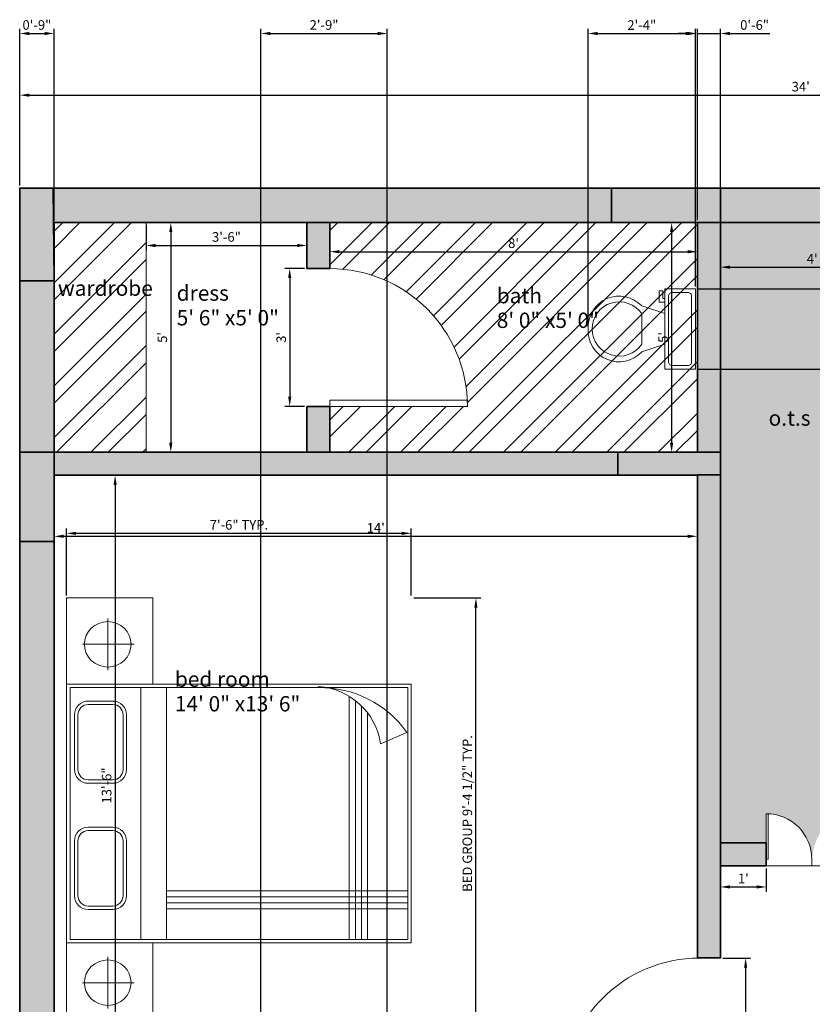
# Model space of a CAD drawing. Units: inches. Extents: x 2369 to 4208, y 1650 to 4492.
# Tile 5 of 6: x 2369 to 2576, y 2257 to 2514. Entities that reach past the tile are written whole.
import ezdxf

# ---------------------------------------------------------------- set-up
doc = ezdxf.new("R2010")
doc.units = ezdxf.units.IN
for name, color, linetype, lineweight in [('A-ANNO-DIMS', 2, 'Continuous', 13), ('A-AREA-IDEN', 7, 'Continuous', 18), ('A-COLS', 7, 'Continuous', 35), ('A-COLS-PATT', 7, 'Continuous', 13), ('A-DOOR', 4, 'Continuous', 18), ('A-FLOR-FIXT', 9, 'Continuous', 18), ('A-FLOR-PATT', 9, 'Continuous', 13), ('A-FURN', 8, 'Continuous', 18), ('A-FURN-FIXD', 8, 'Continuous', 18), ('A-WALL', 7, 'Continuous', 35), ('A-WALL-PATT', 252, 'Continuous', 13)]:
    doc.layers.add(name, color=color, linetype=linetype, lineweight=lineweight)
doc.styles.get("Standard").update_dxf_attribs({"font": 'arial.ttf'})
doc.dimstyles.new('Copy of ISO-25', dxfattribs={"dimtxt": 2.5, "dimasz": 2.5, "dimexe": 1.25, "dimexo": 0.625, "dimtad": 1, "dimdec": 1, "dimlunit": 4, "dimtxsty": 'Standard', "dimcen": 2.5, "dimadec": 0, "dimazin": 0, "dimtfac": 1, "dimtdec": 1, "dimtmove": 0, "dimatfit": 3, "dimfxl": 1, "dimarcsym": 0})

# ---------------------------------------------------------------- blocks, each defined once
blk = doc.blocks.new('*U4')
for p, q in [((-40, 0), (-40, 6)), ((0, 0), (0, 6))]:
    blk.add_line(p, q)
blk.add_lwpolyline([(0, 0), (0, -40), (-1.75, -40), (-1.75, 0)], close=True)
blk.add_arc((0, 0), 40, 180, 270)
blk = doc.blocks.new('*U5')
for p, q in [((0, 0), (0, -6)), ((-40, 0), (-40, -6))]:
    blk.add_line(p, q)
blk.add_lwpolyline([(0, 0), (0, 40), (-1.75, 40), (-1.75, 0)], close=True)
blk.add_arc((0, 0), 40, 90, 180)
blk = doc.blocks.new('*U2')
for p, q in [((0, 0), (0, -6)), ((40, 0), (40, -6))]:
    blk.add_line(p, q)
blk.add_lwpolyline([(0, 0), (0, 40), (1.75, 40), (1.75, 0)], close=True)
blk.add_arc((0, 0), 40, 0, 90)
blk = doc.blocks.new('*D7')
at = {"layer": 'A-ANNO-DIMS', "color": 0, "lineweight": -2, "transparency": 16777216}
for p, q in [((2368.9, 2470.6), (2368.9, 2495.47)), ((2371.4, 2494.22), (2774.4, 2494.22)), ((2776.9, 2470.6), (2776.9, 2495.47))]:
    blk.add_line(p, q, dxfattribs=at)
at = {"layer": 'A-ANNO-DIMS', "color": 0, "transparency": 16777216}
for points in [[(2371.4, 2494.64), (2371.4, 2493.81), (2368.9, 2494.22)], [(2774.4, 2494.64), (2774.4, 2493.81), (2776.9, 2494.22)]]:
    blk.add_solid(points, dxfattribs=at)
at = {"layer": 'Defpoints', "color": 0, "transparency": 16777216}
for p in [(2776.9, 2494.22), (2368.9, 2469.98), (2776.9, 2469.98)]:
    blk.add_point(p, dxfattribs=at)
at = {"layer": 'A-ANNO-DIMS', "color": 0, "transparency": 16777216, "insert": (2572.9, 2496.13), "char_height": 2.5, "attachment_point": 5}
blk.add_mtext("34'", dxfattribs=at)
blk = doc.blocks.new('*D9')
at = {"layer": 'A-ANNO-DIMS', "color": 0, "lineweight": -2, "transparency": 16777216}
for p, q in [((2551.9, 2460.35), (2551.9, 2448.06)), ((2599.9, 2460.35), (2599.9, 2448.06)), ((2554.4, 2449.31), (2597.4, 2449.31))]:
    blk.add_line(p, q, dxfattribs=at)
at = {"layer": 'A-ANNO-DIMS', "color": 0, "transparency": 16777216}
for points in [[(2554.4, 2449.73), (2554.4, 2448.9), (2551.9, 2449.31)], [(2597.4, 2449.73), (2597.4, 2448.9), (2599.9, 2449.31)]]:
    blk.add_solid(points, dxfattribs=at)
at = {"layer": 'Defpoints', "color": 0, "transparency": 16777216}
for p in [(2551.9, 2460.98), (2599.9, 2460.98), (2599.9, 2449.31)]:
    blk.add_point(p, dxfattribs=at)
at = {"layer": 'A-ANNO-DIMS', "color": 0, "transparency": 16777216, "insert": (2575.9, 2451.19), "char_height": 2.5, "attachment_point": 5}
blk.add_mtext("4'", dxfattribs=at)
blk = doc.blocks.new('*D11')
at = {"layer": 'A-ANNO-DIMS', "color": 0, "lineweight": -2, "transparency": 16777216}
for p, q in [((2402.53, 2460.98), (2409.62, 2460.98)), ((2408.37, 2458.48), (2408.37, 2403.48)), ((2402.53, 2400.98), (2409.62, 2400.98))]:
    blk.add_line(p, q, dxfattribs=at)
at = {"layer": 'A-ANNO-DIMS', "color": 0, "transparency": 16777216}
for points in [[(2407.95, 2458.48), (2408.78, 2458.48), (2408.37, 2460.98)], [(2407.95, 2403.48), (2408.78, 2403.48), (2408.37, 2400.98)]]:
    blk.add_solid(points, dxfattribs=at)
at = {"layer": 'Defpoints', "color": 0, "transparency": 16777216}
for p in [(2401.9, 2460.98), (2401.9, 2400.98), (2408.37, 2400.98)]:
    blk.add_point(p, dxfattribs=at)
at = {"layer": 'A-ANNO-DIMS', "color": 0, "transparency": 16777216, "insert": (2406.47, 2430.98), "char_height": 2.5, "attachment_point": 5, "rotation": 90}
blk.add_mtext("5'", dxfattribs=at)
blk = doc.blocks.new('*D12')
at = {"layer": 'A-ANNO-DIMS', "color": 0, "lineweight": -2, "transparency": 16777216}
for p, q in [((2401.9, 2460.35), (2401.9, 2453.73)), ((2443.9, 2460.35), (2443.9, 2453.73)), ((2404.4, 2454.98), (2441.4, 2454.98))]:
    blk.add_line(p, q, dxfattribs=at)
at = {"layer": 'A-ANNO-DIMS', "color": 0, "transparency": 16777216}
for points in [[(2404.4, 2455.4), (2404.4, 2454.56), (2401.9, 2454.98)], [(2441.4, 2455.4), (2441.4, 2454.56), (2443.9, 2454.98)]]:
    blk.add_solid(points, dxfattribs=at)
at = {"layer": 'Defpoints', "color": 0, "transparency": 16777216}
for p in [(2401.9, 2460.98), (2443.9, 2460.98), (2443.9, 2454.98)]:
    blk.add_point(p, dxfattribs=at)
at = {"layer": 'A-ANNO-DIMS', "color": 0, "transparency": 16777216, "insert": (2422.9, 2456.88), "char_height": 2.5, "attachment_point": 5}
blk.add_mtext('3\'-6"', dxfattribs=at)
blk = doc.blocks.new('*D13')
at = {"layer": 'A-ANNO-DIMS', "color": 0, "lineweight": -2, "transparency": 16777216}
for p, q in [((2449.9, 2460.35), (2449.9, 2452.11)), ((2545.9, 2460.35), (2545.9, 2452.11)), ((2452.4, 2453.36), (2543.4, 2453.36))]:
    blk.add_line(p, q, dxfattribs=at)
at = {"layer": 'A-ANNO-DIMS', "color": 0, "transparency": 16777216}
for points in [[(2452.4, 2453.78), (2452.4, 2452.94), (2449.9, 2453.36)], [(2543.4, 2453.78), (2543.4, 2452.94), (2545.9, 2453.36)]]:
    blk.add_solid(points, dxfattribs=at)
at = {"layer": 'Defpoints', "color": 0, "transparency": 16777216}
for p in [(2449.9, 2460.98), (2545.9, 2460.98), (2545.9, 2453.36)]:
    blk.add_point(p, dxfattribs=at)
at = {"layer": 'A-ANNO-DIMS', "color": 0, "transparency": 16777216, "insert": (2497.9, 2455.26), "char_height": 2.5, "attachment_point": 5}
blk.add_mtext("8'", dxfattribs=at)
blk = doc.blocks.new('*D14')
at = {"layer": 'A-ANNO-DIMS', "color": 0, "lineweight": -2, "transparency": 16777216}
for p, q in [((2545.28, 2460.98), (2537.92, 2460.98)), ((2539.17, 2458.48), (2539.17, 2403.48)), ((2545.28, 2400.98), (2537.92, 2400.98))]:
    blk.add_line(p, q, dxfattribs=at)
at = {"layer": 'A-ANNO-DIMS', "color": 0, "transparency": 16777216}
for points in [[(2538.76, 2458.48), (2539.59, 2458.48), (2539.17, 2460.98)], [(2538.76, 2403.48), (2539.59, 2403.48), (2539.17, 2400.98)]]:
    blk.add_solid(points, dxfattribs=at)
at = {"layer": 'Defpoints', "color": 0, "transparency": 16777216}
for p in [(2545.9, 2460.98), (2539.17, 2400.98), (2545.9, 2400.98)]:
    blk.add_point(p, dxfattribs=at)
at = {"layer": 'A-ANNO-DIMS', "color": 0, "transparency": 16777216, "insert": (2537.28, 2430.98), "char_height": 2.5, "attachment_point": 5, "rotation": 90}
blk.add_mtext("5'", dxfattribs=at)
blk = doc.blocks.new('*D19')
at = {"layer": 'A-ANNO-DIMS', "color": 0, "lineweight": -2, "transparency": 16777216}
for p, q in [((2378.53, 2394.98), (2395.08, 2394.98)), ((2393.83, 2392.48), (2393.83, 2235.48)), ((2378.53, 2232.98), (2395.08, 2232.98))]:
    blk.add_line(p, q, dxfattribs=at)
at = {"layer": 'A-ANNO-DIMS', "color": 0, "transparency": 16777216}
for points in [[(2393.41, 2392.48), (2394.24, 2392.48), (2393.83, 2394.98)], [(2393.41, 2235.48), (2394.24, 2235.48), (2393.83, 2232.98)]]:
    blk.add_solid(points, dxfattribs=at)
at = {"layer": 'Defpoints', "color": 0, "transparency": 16777216}
for p in [(2377.9, 2394.98), (2377.9, 2232.98), (2393.83, 2232.98)]:
    blk.add_point(p, dxfattribs=at)
at = {"layer": 'A-ANNO-DIMS', "color": 0, "transparency": 16777216, "insert": (2391.93, 2313.98), "char_height": 2.5, "attachment_point": 5, "rotation": 90}
blk.add_mtext('13\'-6"', dxfattribs=at)
blk = doc.blocks.new('*D20')
at = {"layer": 'A-ANNO-DIMS', "color": 0, "lineweight": -2, "transparency": 16777216}
for p, q in [((2377.9, 2394.35), (2377.9, 2377.8)), ((2545.9, 2394.35), (2545.9, 2377.8)), ((2380.4, 2379.05), (2543.4, 2379.05))]:
    blk.add_line(p, q, dxfattribs=at)
at = {"layer": 'A-ANNO-DIMS', "color": 0, "transparency": 16777216}
for points in [[(2380.4, 2379.47), (2380.4, 2378.63), (2377.9, 2379.05)], [(2543.4, 2379.47), (2543.4, 2378.63), (2545.9, 2379.05)]]:
    blk.add_solid(points, dxfattribs=at)
at = {"layer": 'Defpoints', "color": 0, "transparency": 16777216}
for p in [(2377.9, 2394.98), (2545.9, 2394.98), (2545.9, 2379.05)]:
    blk.add_point(p, dxfattribs=at)
at = {"layer": 'A-ANNO-DIMS', "color": 0, "transparency": 16777216, "insert": (2461.9, 2380.93), "char_height": 2.5, "attachment_point": 5}
blk.add_mtext("14'", dxfattribs=at)
blk = doc.blocks.new('A$C057D194F')
for p, q in [((0, 1.5, -0.1688), (0, 2, -0.1688)), ((0, 2, -0.1688), (0.5, 2, -0.1688)), ((0.5, 2, -0.1688), (0.5, 0, -0.1688)), ((2, 2, -0.1688), (0.5, 2, -0.1688)), ((2, 0, -0.1688), (2, 2, -0.1688)), ((2.5, 2, -0.1688), (2, 2, -0.1688)), ((2.5, 1.5, -0.1688), (2.5, 2, -0.1688)), ((1.98, 1.98, -0.1688), (0.52, 1.98, -0.1688)), ((0.52, 1.98, -0.1688), (0.52, 0.02, -0.1688)), ((1.0907, 1.9539, -0.1688), (0.7735, 1.9539, -0.1688)), ((1.8224, 1.9539, -0.1688), (1.5052, 1.9539, -0.1688)), ((1.98, 0.02, -0.1688), (1.98, 1.98, -0.1688)), ((0.2687, 1.9081, -0.1688), (0.2687, 1.761, -0.1688)), ((0.2687, 1.6081, -0.1688), (0.2687, 1.9081, -0.1688)), ((1.0907, 1.9339, -0.1688), (0.7735, 1.9339, -0.1688)), ((1.8224, 1.9339, -0.1688), (1.5052, 1.9339, -0.1688)), ((2.2313, 1.9081, -0.1688), (2.2313, 1.761, -0.1688)), ((2.2313, 1.6081, -0.1688), (2.2313, 1.9081, -0.1688)), ((0.6935, 1.8739, -0.1688), (0.6935, 1.7322, -0.1688)), ((0.7135, 1.8739, -0.1688), (0.7135, 1.7322, -0.1688)), ((1.1507, 1.7322, -0.1688), (1.1507, 1.8739, -0.1688)), ((1.1707, 1.7322, -0.1688), (1.1707, 1.8739, -0.1688)), ((1.4252, 1.8739, -0.1688), (1.4252, 1.7322, -0.1688)), ((1.4452, 1.8739, -0.1688), (1.4452, 1.7322, -0.1688)), ((1.8824, 1.7322, -0.1688), (1.8824, 1.8739, -0.1688)), ((1.9024, 1.7322, -0.1688), (1.9024, 1.8739, -0.1688)), ((0.4194, 1.761, -0.1688), (0.1194, 1.761, -0.1688)), ((0.2687, 1.761, -0.1688), (0.4194, 1.761, -0.1688)), ((0.2687, 1.761, -0.1688), (0.2687, 1.6081, -0.1688)), ((2.0806, 1.761, -0.1688), (2.3806, 1.761, -0.1688)), ((2.2313, 1.761, -0.1688), (2.0806, 1.761, -0.1688)), ((2.2313, 1.761, -0.1688), (2.2313, 1.6081, -0.1688)), ((0.7735, 1.6722, -0.1688), (1.0907, 1.6722, -0.1688)), ((1.5052, 1.6722, -0.1688), (1.8224, 1.6722, -0.1688)), ((0.7735, 1.6522, -0.1688), (1.0907, 1.6522, -0.1688)), ((1.5052, 1.6522, -0.1688), (1.8224, 1.6522, -0.1688)), ((1.98, 1.5693, -0.1688), (0.52, 1.5693, -0.1688)), ((0.5, 1.5, -0.1688), (0, 1.5, -0.1688)), ((2, 1.5, -0.1688), (2.5, 1.5, -0.1688)), ((1.98, 1.4193, -0.1688), (0.52, 1.4193, -0.1688)), ((0.6969, 0.02, -0.1688), (0.6969, 1.4193, -0.1688)), ((0.7319, 0.02, -0.1688), (0.7319, 1.4193, -0.1688)), ((0.7669, 0.02, -0.1688), (0.7669, 1.4193, -0.1688)), ((0.8019, 0.02, -0.1688), (0.8019, 1.4193, -0.1688)), ((0.52, 0.3595, -0.1688), (1.9292, 0.3595, -0.1688)), ((0.52, 0.3245, -0.1688), (1.905, 0.3245, -0.1688)), ((0.52, 0.2895, -0.1688), (1.8742, 0.2895, -0.1688)), ((0.52, 0.2545, -0.1688), (1.8344, 0.2545, -0.1688)), ((1.6548, 0.1789, -0.1688), (1.7198, 0.0251, -0.1688)), ((0.52, 0.02, -0.1688), (1.98, 0.02, -0.1688)), ((0.5, 0, -0.1688), (2, 0, -0.1688))]:
    blk.add_line(p, q)
for centre, radius, start, end in [((0.7735, 1.8739, -0.1688), 0.08, 90, 180), ((1.0907, 1.8739, -0.1688), 0.08, 0, 90), ((1.5052, 1.8739, -0.1688), 0.08, 90, 180), ((1.8224, 1.8739, -0.1688), 0.08, 0, 90), ((0.7735, 1.8739, -0.1688), 0.06, 90, 180), ((1.0907, 1.8739, -0.1688), 0.06, 0, 90), ((1.5052, 1.8739, -0.1688), 0.06, 90, 180), ((1.8224, 1.8739, -0.1688), 0.06, 0, 90), ((0.7735, 1.7322, -0.1688), 0.08, 180, 270), ((0.7735, 1.7322, -0.1688), 0.06, 180, 270), ((1.0907, 1.7322, -0.1688), 0.08, 270, 0), ((1.0907, 1.7322, -0.1688), 0.06, 270, 0), ((1.5052, 1.7322, -0.1688), 0.08, 180, 270), ((1.5052, 1.7322, -0.1688), 0.06, 180, 270), ((1.8224, 1.7322, -0.1688), 0.08, 270, 0), ((1.8224, 1.7322, -0.1688), 0.06, 270, 0), ((1.5992, 0.5623, -0.1688), 0.3874, 278.2518, 356.6808), ((1.363, 0.5286, -0.1688), 0.6171, 305.3295, 1.0459)]:
    blk.add_arc(centre, radius, start, end)
blk.add_ellipse((0.2687, 1.761, -0.1688), major_axis=(0, -0.1351), ratio=0.975448)
at = {"extrusion": (0, 0, -1)}
blk.add_ellipse((2.2313, 1.761, -0.1688), major_axis=(0, 0.1351), ratio=0.975448, dxfattribs=at)
for p in [(0.2687, 1.761, -0.1688), (2.2313, 1.761, -0.1688)]:
    blk.add_point(p)
blk = doc.blocks.new('*D38')
at = {"layer": 'A-ANNO-DIMS', "color": 0, "lineweight": -2, "transparency": 16777216}
for p, q in [((2552.53, 2268.93), (2559.75, 2268.93)), ((2558.5, 2266.43), (2558.5, 2235.48)), ((2552.53, 2232.98), (2559.75, 2232.98))]:
    blk.add_line(p, q, dxfattribs=at)
at = {"layer": 'A-ANNO-DIMS', "color": 0, "transparency": 16777216}
for points in [[(2558.09, 2266.43), (2558.92, 2266.43), (2558.5, 2268.93)], [(2558.09, 2235.48), (2558.92, 2235.48), (2558.5, 2232.98)]]:
    blk.add_solid(points, dxfattribs=at)
at = {"layer": 'Defpoints', "color": 0, "transparency": 16777216}
for p in [(2551.9, 2268.93), (2551.9, 2232.98), (2558.5, 2232.98)]:
    blk.add_point(p, dxfattribs=at)
at = {"layer": 'A-ANNO-DIMS', "color": 0, "transparency": 16777216, "insert": (2556.6, 2250.95), "char_height": 2.5, "attachment_point": 5, "rotation": 90}
blk.add_mtext("3'", dxfattribs=at)
blk = doc.blocks.new('*D39')
at = {"layer": 'A-ANNO-DIMS', "color": 0, "lineweight": -2, "transparency": 16777216}
for p, q in [((2551.9, 2292.35), (2551.9, 2286.25)), ((2563.9, 2292.35), (2563.9, 2286.25)), ((2554.4, 2287.5), (2561.4, 2287.5))]:
    blk.add_line(p, q, dxfattribs=at)
at = {"layer": 'A-ANNO-DIMS', "color": 0, "transparency": 16777216}
for points in [[(2554.4, 2287.92), (2554.4, 2287.08), (2551.9, 2287.5)], [(2561.4, 2287.92), (2561.4, 2287.08), (2563.9, 2287.5)]]:
    blk.add_solid(points, dxfattribs=at)
at = {"layer": 'Defpoints', "color": 0, "transparency": 16777216}
for p in [(2551.9, 2292.98), (2563.9, 2292.98), (2563.9, 2287.5)]:
    blk.add_point(p, dxfattribs=at)
at = {"layer": 'A-ANNO-DIMS', "color": 0, "transparency": 16777216, "insert": (2557.9, 2289.38), "char_height": 2.5, "attachment_point": 5}
blk.add_mtext("1'", dxfattribs=at)
blk = doc.blocks.new('*D42')
at = {"layer": 'A-ANNO-DIMS', "color": 0, "lineweight": -2, "transparency": 16777216}
for p, q in [((2443.28, 2448.98), (2438.17, 2448.98)), ((2439.42, 2446.48), (2439.42, 2415.48)), ((2443.28, 2412.98), (2438.17, 2412.98))]:
    blk.add_line(p, q, dxfattribs=at)
at = {"layer": 'A-ANNO-DIMS', "color": 0, "transparency": 16777216}
for points in [[(2439.01, 2446.48), (2439.84, 2446.48), (2439.42, 2448.98)], [(2439.01, 2415.48), (2439.84, 2415.48), (2439.42, 2412.98)]]:
    blk.add_solid(points, dxfattribs=at)
at = {"layer": 'Defpoints', "color": 0, "transparency": 16777216}
for p in [(2443.9, 2448.98), (2439.42, 2412.98), (2443.9, 2412.98)]:
    blk.add_point(p, dxfattribs=at)
at = {"layer": 'A-ANNO-DIMS', "color": 0, "transparency": 16777216, "insert": (2437.52, 2430.98), "char_height": 2.5, "attachment_point": 5, "rotation": 90}
blk.add_mtext("3'", dxfattribs=at)
blk = doc.blocks.new('*U47')
for p, q in [((241.3, -152.4), (241.3, -50.8)), ((-254, -215.9), (-203.2, -215.9)), ((-254, -241.3), (-254, -215.9)), ((-177.8, -241.3), (-254, -241.3)), ((-203.2, -215.9), (-203.2, -203.2)), ((-177.8, -203.2), (-177.8, -241.3)), ((-101.6, -203.2), (-152.4, -355.6)), ((101.6, -203.2), (152.4, -355.6)), ((101.6, -355.6), (-101.6, -355.6))]:
    blk.add_line(p, q)
blk.add_lwpolyline([(266.7, -203.2), (266.7, 0), (-266.7, 0), (-266.7, -203.2)], close=True)
for points in [[(-241.3, -50.8), (-241.3, -152.4)], [(215.9, -25.4), (-215.9, -25.4)], [(-215.9, -177.8), (215.9, -177.8)]]:
    blk.add_lwpolyline(points)
for centre, radius, start, end in [((-219.075, -47.625), 22.45064, 81.8699, 188.1301), ((219.075, -47.625), 22.45064, 351.8699, 98.1301), ((-219.075, -155.575), 22.45064, 171.869898, 278.1301), ((219.075, -155.575), 22.45064, 261.8699, 8.1301), ((-12.12088, -505.93752), 205.61935, 133.01722, 273.38), ((0.94996, -504.77674), 181.02486, 124.50543, 269.7), ((-0.94742, -504.77674), 181.02486, 270.3, 55.4946), ((12.12342, -505.93752), 205.61935, 266.62, 46.9828)]:
    blk.add_arc(centre, radius, start, end)
blk = doc.blocks.new('*D49')
at = {"layer": 'A-ANNO-DIMS', "color": 0, "lineweight": -2, "transparency": 16777216}
for p, q in [((2471.81, 2362.94), (2489.31, 2362.94)), ((2488.06, 2252.9), (2488.06, 2360.44)), ((2471.81, 2250.4), (2489.31, 2250.4))]:
    blk.add_line(p, q, dxfattribs=at)
at = {"layer": 'A-ANNO-DIMS', "color": 0, "transparency": 16777216}
for points in [[(2487.64, 2360.44), (2488.48, 2360.44), (2488.06, 2362.94)], [(2487.64, 2252.9), (2488.48, 2252.9), (2488.06, 2250.4)]]:
    blk.add_solid(points, dxfattribs=at)
at = {"layer": 'Defpoints', "color": 0, "transparency": 16777216}
for p in [(2471.18, 2362.94), (2488.06, 2362.94), (2471.18, 2250.4)]:
    blk.add_point(p, dxfattribs=at)
at = {"layer": 'A-ANNO-DIMS', "color": 0, "transparency": 16777216, "insert": (2486.14, 2306.67), "char_height": 2.5, "attachment_point": 5, "rotation": 90}
blk.add_mtext('BED GROUP 9\'-4 1/2" TYP.', dxfattribs=at)
blk = doc.blocks.new('*D50')
at = {"layer": 'A-ANNO-DIMS', "color": 0, "lineweight": -2, "transparency": 16777216}
for p, q in [((2381.15, 2363.56), (2381.15, 2381.07)), ((2471.18, 2363.56), (2471.18, 2381.07)), ((2468.68, 2379.82), (2383.65, 2379.82))]:
    blk.add_line(p, q, dxfattribs=at)
at = {"layer": 'A-ANNO-DIMS', "color": 0, "transparency": 16777216}
for points in [[(2383.65, 2380.24), (2383.65, 2379.4), (2381.15, 2379.82)], [(2468.68, 2380.24), (2468.68, 2379.4), (2471.18, 2379.82)]]:
    blk.add_solid(points, dxfattribs=at)
at = {"layer": 'Defpoints', "color": 0, "transparency": 16777216}
for p in [(2381.15, 2379.82), (2381.15, 2362.94), (2471.18, 2362.94)]:
    blk.add_point(p, dxfattribs=at)
at = {"layer": 'A-ANNO-DIMS', "color": 0, "transparency": 16777216, "insert": (2426.16, 2381.72), "char_height": 2.5, "attachment_point": 5}
blk.add_mtext('7\'-6" TYP.', dxfattribs=at)
blk = doc.blocks.new('*D61')
at = {"layer": 'A-ANNO-DIMS', "color": 0, "lineweight": -2, "transparency": 16777216}
for p, q in [((2431.9, 2100.6), (2431.9, 2511.58)), ((2434.4, 2510.33), (2462.4, 2510.33)), ((2464.9, 2100.6), (2464.9, 2511.58))]:
    blk.add_line(p, q, dxfattribs=at)
at = {"layer": 'A-ANNO-DIMS', "color": 0, "transparency": 16777216}
for points in [[(2434.4, 2510.75), (2434.4, 2509.91), (2431.9, 2510.33)], [(2462.4, 2510.75), (2462.4, 2509.91), (2464.9, 2510.33)]]:
    blk.add_solid(points, dxfattribs=at)
at = {"layer": 'Defpoints', "color": 0, "transparency": 16777216}
for p in [(2464.9, 2510.33), (2431.9, 2099.98), (2464.9, 2099.98)]:
    blk.add_point(p, dxfattribs=at)
at = {"layer": 'A-ANNO-DIMS', "color": 0, "transparency": 16777216, "insert": (2448.4, 2512.23), "char_height": 2.5, "attachment_point": 5}
blk.add_mtext('2\'-9"', dxfattribs=at)
blk = doc.blocks.new('*D62')
at = {"layer": 'A-ANNO-DIMS', "color": 0, "lineweight": -2, "transparency": 16777216}
for p, q in [((2517.38, 2433.8), (2517.38, 2511.58)), ((2519.88, 2510.33), (2542.88, 2510.33)), ((2545.38, 2444.3), (2545.38, 2511.58))]:
    blk.add_line(p, q, dxfattribs=at)
at = {"layer": 'A-ANNO-DIMS', "color": 0, "transparency": 16777216}
for points in [[(2519.88, 2510.75), (2519.88, 2509.91), (2517.38, 2510.33)], [(2542.88, 2510.75), (2542.88, 2509.91), (2545.38, 2510.33)]]:
    blk.add_solid(points, dxfattribs=at)
at = {"layer": 'Defpoints', "color": 0, "transparency": 16777216}
for p in [(2545.38, 2510.33), (2545.38, 2443.68), (2517.38, 2433.18)]:
    blk.add_point(p, dxfattribs=at)
at = {"layer": 'A-ANNO-DIMS', "color": 0, "transparency": 16777216, "insert": (2531.38, 2512.21), "char_height": 2.5, "attachment_point": 5}
blk.add_mtext('2\'-4"', dxfattribs=at)
blk = doc.blocks.new('*D63')
at = {"layer": 'A-ANNO-DIMS', "color": 0, "lineweight": -2, "transparency": 16777216}
for p, q in [((2546, 2443.68), (2818.5, 2443.68)), ((2817.25, 2441.18), (2817.25, 2425.18)), ((2546, 2422.68), (2818.5, 2422.68))]:
    blk.add_line(p, q, dxfattribs=at)
at = {"layer": 'A-ANNO-DIMS', "color": 0, "transparency": 16777216}
for points in [[(2816.83, 2441.18), (2817.67, 2441.18), (2817.25, 2443.68)], [(2816.83, 2425.18), (2817.67, 2425.18), (2817.25, 2422.68)]]:
    blk.add_solid(points, dxfattribs=at)
at = {"layer": 'Defpoints', "color": 0, "transparency": 16777216}
for p in [(2545.38, 2443.68), (2545.38, 2422.68), (2817.25, 2422.68)]:
    blk.add_point(p, dxfattribs=at)
at = {"layer": 'A-ANNO-DIMS', "color": 0, "transparency": 16777216, "insert": (2815.35, 2433.18), "char_height": 2.5, "attachment_point": 5, "rotation": 90}
blk.add_mtext('1\'-9"', dxfattribs=at)
blk = doc.blocks.new('*D64')
at = {"layer": 'A-ANNO-DIMS', "color": 0, "lineweight": -2, "transparency": 16777216}
for p, q in [((2543.4, 2510.33), (2540.9, 2510.33)), ((2545.9, 2461.6), (2545.9, 2511.58)), ((2545.9, 2510.33), (2551.9, 2510.33)), ((2551.9, 2461.6), (2551.9, 2511.58)), ((2554.4, 2510.33), (2564.8, 2510.33))]:
    blk.add_line(p, q, dxfattribs=at)
at = {"layer": 'A-ANNO-DIMS', "color": 0, "transparency": 16777216}
for points in [[(2543.4, 2510.75), (2543.4, 2509.91), (2545.9, 2510.33)], [(2554.4, 2510.75), (2554.4, 2509.91), (2551.9, 2510.33)]]:
    blk.add_solid(points, dxfattribs=at)
at = {"layer": 'Defpoints', "color": 0, "transparency": 16777216}
for p in [(2551.9, 2510.33), (2545.9, 2460.98), (2551.9, 2460.98)]:
    blk.add_point(p, dxfattribs=at)
at = {"layer": 'A-ANNO-DIMS', "color": 0, "transparency": 16777216, "insert": (2560.85, 2512.23), "char_height": 2.5, "attachment_point": 5}
blk.add_mtext('0\'-6"', dxfattribs=at)
blk = doc.blocks.new('*D65')
at = {"layer": 'A-ANNO-DIMS', "color": 0, "lineweight": -2, "transparency": 16777216}
for p, q in [((2368.9, 2470.6), (2368.9, 2511.58)), ((2371.4, 2510.33), (2375.4, 2510.33)), ((2377.9, 2461.6), (2377.9, 2511.58))]:
    blk.add_line(p, q, dxfattribs=at)
at = {"layer": 'A-ANNO-DIMS', "color": 0, "transparency": 16777216}
for points in [[(2371.4, 2510.75), (2371.4, 2509.91), (2368.9, 2510.33)], [(2375.4, 2510.75), (2375.4, 2509.91), (2377.9, 2510.33)]]:
    blk.add_solid(points, dxfattribs=at)
at = {"layer": 'Defpoints', "color": 0, "transparency": 16777216}
for p in [(2377.9, 2510.33), (2368.9, 2469.98), (2377.9, 2460.98)]:
    blk.add_point(p, dxfattribs=at)
at = {"layer": 'A-ANNO-DIMS', "color": 0, "transparency": 16777216, "insert": (2373.4, 2512.23), "char_height": 2.5, "attachment_point": 5}
blk.add_mtext('0\'-9"', dxfattribs=at)

msp = doc.modelspace()

# ---------------------------------------------------------------- hatches: boundary and pattern name
at = {"layer": 'A-COLS-PATT'}
h = msp.add_hatch(color=256, dxfattribs=at)
h.dxf.hatch_style = 1
h.paths.add_polyline_path([(2377.9, 2254.21), (2368.9, 2254.21), (2368.9, 2226.98), (2377.9, 2226.98)])
h.paths.add_polyline_path([(2551.9, 2400.98), (2545.9, 2400.98), (2525.15, 2400.98), (2525.15, 2394.98), (2545.9, 2395.12), (2551.9, 2395.12)])
h.paths.add_polyline_path([(2637.99, 2400.98), (2599.9, 2400.98), (2599.9, 2394.98), (2605.9, 2394.98), (2637.99, 2394.98)])
h.paths.add_polyline_path([(2623.27, 2232.98), (2599.9, 2232.98), (2599.9, 2226.98), (2623.27, 2226.98)])
h.paths.add_polyline_path([(2551.9, 2232.98), (2528.53, 2232.98), (2528.53, 2226.98), (2551.9, 2226.98)])
h.paths.add_polyline_path([(2731.9, 2232.98), (2713.81, 2232.98), (2713.81, 2226.98), (2731.9, 2226.98)])
h.paths.add_polyline_path([(2776.9, 2250.53), (2767.9, 2250.53), (2767.9, 2232.98), (2767.9, 2226.98), (2776.9, 2226.98)])
h.paths.add_polyline_path([(2776.9, 2078.3), (2767.9, 2078.3), (2767.9, 2058.98), (2767.9, 2052.98), (2776.9, 2052.98)])
h.paths.add_polyline_path([(2731.9, 2058.98), (2725.9, 2058.98), (2713.81, 2058.98), (2713.81, 2052.98), (2731.9, 2052.98)])
h.paths.add_polyline_path([(2776.9, 1973.96), (2767.9, 1973.96), (2767.9, 1956.98), (2767.9, 1950.98), (2776.9, 1950.98)])
h.paths.add_polyline_path([(2776.9, 1775.33), (2767.9, 1775.33), (2767.9, 1758.98), (2767.9, 1749.98), (2776.9, 1749.98)])
h.paths.add_polyline_path([(2569.9, 1758.98), (2560.9, 1758.98), (2560.9, 1749.98), (2569.9, 1749.98)])
h.paths.add_polyline_path([(2377.9, 1774.03), (2368.9, 1774.03), (2368.9, 1749.98), (2372.9, 1749.98), (2377.9, 1749.98)])
h.paths.add_polyline_path([(2377.9, 1926.53), (2368.9, 1926.53), (2368.9, 1902.98), (2377.9, 1902.98)])
h.paths.add_polyline_path([(2377.9, 2079.34), (2368.9, 2079.34), (2368.9, 2052.98), (2377.9, 2052.98), (2377.9, 2057.9)])
at = {"layer": 'A-FLOR-PATT'}
h = msp.add_hatch(dxfattribs=at)
h.set_pattern_fill('ANSI32', color=256)
h.paths.add_polyline_path([(2545.9, 2460.98), (2523.46, 2460.98), (2449.9, 2460.98), (2449.9, 2448.93, -0.401453), (2485.82, 2414.55), (2485.85, 2414.55), (2485.85, 2412.98), (2449.9, 2412.98), (2449.9, 2400.98), (2545.9, 2400.98)])
h.paths.add_polyline_path([(2701.9, 2448.92), (2701.9, 2460.98), (2605.9, 2460.98), (2605.9, 2400.98), (2637.99, 2400.98), (2701.9, 2400.98), (2701.9, 2412.98), (2666.56, 2412.98), (2666.56, 2414.55), (2666.59, 2414.55, -0.396556)])
h.paths.add_polyline_path([(2425.9, 2148.98), (2377.9, 2148.98), (2377.9, 2090.68), (2379.33, 2090.68), (2379.33, 2090.65, -0.391899), (2410.67, 2058.98), (2425.9, 2058.98), (2425.9, 2094.98), (2425.9, 2100.98)])
h.paths.add_polyline_path([(2401.9, 2460.98), (2377.9, 2460.98), (2377.9, 2400.98), (2401.9, 2400.98)])
h.paths.add_polyline_path([(2767.9, 2460.98), (2743.9, 2460.98), (2743.9, 2400.98), (2767.9, 2400.98)])
h.paths.add_polyline_path([(2767.9, 2226.98), (2731.9, 2226.98), (2731.9, 2058.98), (2767.9, 2058.98)])
h.paths.add_polyline_path([(2612.47, 2434.38), (2640.5, 2434.38), (2640.5, 2440.51), (2612.47, 2440.51)], flags=24)
h.paths.add_polyline_path([(2612.48, 2440.81), (2625.39, 2440.81), (2625.39, 2446.91), (2612.48, 2446.91)], flags=24)
h.paths.add_polyline_path([(2712.27, 2432.83), (2738.74, 2432.83), (2738.74, 2438.96), (2712.27, 2438.96)], flags=9)
h.paths.add_polyline_path([(2712.27, 2439.27), (2727.97, 2439.27), (2727.97, 2445.37), (2712.27, 2445.37)], flags=9)
h.paths.add_polyline_path([(2492.48, 2432.36), (2520.5, 2432.36), (2520.5, 2438.49), (2492.48, 2438.49)], flags=24)
h.paths.add_polyline_path([(2492.48, 2438.8), (2505.39, 2438.8), (2505.39, 2444.9), (2492.48, 2444.9)], flags=24)
h.paths.add_polyline_path([(2386, 2119.22), (2414.03, 2119.22), (2414.03, 2125.35), (2386, 2125.35)], flags=24)
h.paths.add_polyline_path([(2386.01, 2125.66), (2398.92, 2125.66), (2398.92, 2131.75), (2386.01, 2131.75)], flags=24)
h.paths.add_polyline_path([(2377.88, 2440.75), (2403.21, 2440.75), (2403.21, 2446.85), (2377.88, 2446.85)], flags=9)
h.paths.add_polyline_path([(2743.66, 2441.21), (2768.99, 2441.21), (2768.99, 2447.31), (2743.66, 2447.31)], flags=9)
h.paths.add_polyline_path([(2739.13, 2166.12), (2752.65, 2166.12), (2752.65, 2172.22), (2739.13, 2172.22)], flags=24)
h.paths.add_polyline_path([(2739.12, 2172.54), (2751.98, 2172.54), (2751.98, 2178.67), (2739.12, 2178.67)], flags=24)
h.paths.add_polyline_path([(2738.85, 2177.59), (2749.82, 2177.59), (2749.82, 2185.35), (2738.85, 2185.35)], flags=24)
h.paths.add_polyline_path([(2739.15, 2185.42), (2747.35, 2185.42), (2747.35, 2191.39), (2739.15, 2191.39)], flags=24)
h.paths.add_polyline_path([(2739.12, 2190.78), (2753.59, 2190.78), (2753.59, 2196.89), (2739.12, 2196.89)], flags=24)
h = msp.add_hatch(dxfattribs=at)
h.set_pattern_fill('ANGLE', color=256)
h.set_pattern_definition([(0, (0, 0), (0, 6.985), [5.08, -1.905]), (90, (0, 0), (-6.985, 4e-16), [5.08, -1.905])])
h.paths.add_polyline_path([(2599.9, 2460.98), (2551.9, 2460.98), (2551.9, 2298.98), (2563.9, 2298.98), (2563.9, 2306.63), (2564.42, 2306.63), (2564.42, 2306.61, -0.405418), (2575.94, 2294.77, -0.401619), (2587.38, 2306.72), (2587.38, 2306.73), (2587.9, 2306.73), (2587.9, 2298.98), (2599.9, 2298.98)])
h.paths.add_polyline_path([(2425.9, 2226.98), (2377.9, 2226.98), (2377.9, 2154.98), (2389.9, 2154.98), (2425.9, 2154.98)])
h.paths.add_polyline_path([(2641.9, 2052.98), (2569.9, 2052.98), (2569.9, 1998.98), (2581.9, 1998.98), (2581.9, 1992.98), (2606.44, 1992.98), (2629.9, 1992.98), (2629.9, 1998.98), (2641.9, 1998.98), (2641.9, 2008.36), (2647.9, 2008.36), (2647.9, 1956.98), (2767.9, 1956.98), (2767.9, 2052.98), (2647.9, 2052.98), (2647.9, 2044.36), (2641.9, 2044.36)])
h.paths.add_polyline_path([(2628.69, 2019.73), (2629.71, 2019.73), (2629.71, 1996.47), (2628.69, 1996.47)], flags=16)
h.paths.add_polyline_path([(2563.51, 2406.86), (2576.05, 2406.86), (2576.05, 2412.82), (2563.51, 2412.82)], flags=24)
h.paths.add_polyline_path([(2391.33, 2190.25), (2403.87, 2190.25), (2403.87, 2196.21), (2391.33, 2196.21)], flags=24)
h.paths.add_polyline_path([(2704.89, 2039.23), (2710.69, 2039.23), (2710.69, 2044.38), (2704.89, 2044.38)], flags=24)
h.paths.add_polyline_path([(2759.77, 2003.06), (2759.77, 2006.92), (2754.62, 2006.92), (2754.62, 2003.06)], flags=24)
h.paths.add_polyline_path([(2707.15, 2003.75), (2738.28, 2003.75), (2738.28, 2009.88), (2707.15, 2009.88)], flags=24)
h.paths.add_polyline_path([(2707.15, 2010.19), (2726.89, 2010.19), (2726.89, 2016.29), (2707.15, 2016.29)], flags=24)
h.paths.add_polyline_path([(2577.31, 2031), (2605.34, 2031), (2605.34, 2037.12), (2577.31, 2037.12)], flags=24)
h.paths.add_polyline_path([(2577.02, 2036.02), (2603.33, 2036.02), (2603.33, 2043.89), (2577.02, 2043.89)], flags=24)
at = {"layer": 'A-WALL-PATT'}
h = msp.add_hatch(color=256, dxfattribs=at)
h.dxf.hatch_style = 1
h.paths.add_polyline_path([(2377.9, 2052.98), (2368.9, 2052.98), (2368.9, 1926.53), (2377.9, 1926.53)])
h.paths.add_polyline_path([(2377.9, 2226.98), (2368.9, 2226.98), (2368.9, 2079.34), (2377.9, 2079.34)])
h.paths.add_polyline_path([(2377.9, 2394.98), (2377.9, 2460.98), (2767.9, 2460.98), (2767.9, 2250.53), (2776.9, 2250.53), (2776.9, 2469.98), (2368.9, 2469.98), (2368.9, 2254.21), (2377.9, 2254.21)])
h.paths.add_polyline_path([(2776.9, 2226.98), (2767.9, 2226.98), (2767.9, 2078.3), (2776.9, 2078.3)])
h.paths.add_polyline_path([(2776.9, 2052.98), (2767.9, 2052.98), (2767.9, 1973.96), (2776.9, 1973.96)])
h.paths.add_polyline_path([(2776.9, 1950.98), (2767.9, 1950.98), (2767.9, 1775.33), (2776.9, 1775.33)])
h.paths.add_polyline_path([(2560.9, 1758.98), (2377.9, 1758.98), (2377.9, 1749.98), (2386.24, 1749.98), (2386.07, 1750.89), (2387.22, 1749.98), (2560.9, 1749.98)])
h.paths.add_polyline_path([(2377.9, 1902.98), (2368.9, 1902.98), (2368.9, 1774.03), (2377.9, 1774.03)])
h.paths.add_polyline_path([(2569.9, 1908.98), (2569.9, 1944.98), (2563.9, 1944.98), (2563.9, 1908.98), (2377.9, 1908.98), (2377.9, 1902.98), (2569.9, 1902.98)])
h.paths.add_polyline_path([(2523.29, 2058.98), (2411, 2058.98), (2411, 2052.98), (2523.29, 2052.98)])
h.paths.add_polyline_path([(2569.9, 2052.98), (2641.9, 2052.98), (2713.81, 2052.98), (2713.81, 2058.98), (2559.29, 2058.98), (2559.29, 2052.98), (2563.9, 2052.98), (2563.9, 1980.98), (2569.9, 1980.98), (2569.9, 1992.98)])
h.paths.add_polyline_path([(2528.53, 2232.98), (2510.56, 2232.98), (2377.9, 2232.98), (2377.9, 2226.98), (2528.53, 2226.98)])
h.paths.add_polyline_path([(2713.81, 2232.98), (2623.27, 2232.98), (2623.27, 2226.98), (2713.81, 2226.98)])
h.paths.add_polyline_path([(2647.9, 2008.36), (2642.51, 2008.36), (2641.9, 2008.36), (2641.9, 1956.98), (2641.9, 1950.98), (2767.9, 1950.98), (2767.9, 1956.98), (2647.9, 1956.98)])
h.paths.add_polyline_path([(2551.9, 2395.12), (2545.9, 2395.12), (2545.9, 2268.98), (2551.9, 2268.98)], flags=17)
h.paths.add_polyline_path([(2551.9, 2460.98), (2545.9, 2460.98), (2545.9, 2400.98), (2551.9, 2400.98)], flags=17)
h.paths.add_polyline_path([(2605.9, 2460.98), (2599.9, 2460.98), (2599.9, 2400.98), (2605.9, 2400.98)], flags=17)
h.paths.add_polyline_path([(2767.9, 2400.98), (2637.99, 2400.98), (2637.99, 2394.98), (2767.9, 2394.98)], flags=17)
h.paths.add_polyline_path([(2605.9, 2394.98), (2599.9, 2394.98), (2599.9, 2394.42), (2599.9, 2268.98), (2605.9, 2268.98)], flags=17)
h.paths.add_polyline_path([(2525.15, 2400.98), (2377.9, 2400.98), (2377.9, 2394.98), (2525.15, 2394.98)], flags=17)
h.paths.add_polyline_path([(2449.9, 2412.98), (2444.51, 2412.98), (2443.9, 2412.98), (2443.9, 2400.98), (2449.9, 2400.98)], flags=17)
h.paths.add_polyline_path([(2449.9, 2460.98), (2443.9, 2460.98), (2443.9, 2448.98), (2449.9, 2448.98)], flags=17)
h.paths.add_polyline_path([(2731.9, 2106.98), (2725.9, 2106.98), (2725.9, 2058.98), (2731.9, 2058.98)])
h = msp.add_hatch(color=256, dxfattribs=at)
h.dxf.hatch_style = 1
h.paths.add_polyline_path([(2563.9, 2294.76), (2563.9, 2298.98), (2551.9, 2298.98), (2551.9, 2292.98), (2563.9, 2292.98)])
h.paths.add_polyline_path([(2599.9, 2298.98), (2587.9, 2298.98), (2587.9, 2294.77), (2587.9, 2292.98), (2599.9, 2292.98)])

# ---------------------------------------------------------------- linework, layer by layer
at = {"layer": 'A-COLS'}
for p, q in [((2368.9, 2469.98), (2377.66, 2469.98)), ((2377.66, 2469.98), (2377.9, 2445.74)), ((2551.9, 2469.98), (2523.46, 2469.98)), ((2523.46, 2469.98), (2523.46, 2460.98)), ((2551.9, 2460.98), (2551.9, 2469.98)), ((2523.46, 2460.98), (2551.9, 2460.98)), ((2377.9, 2445.74), (2368.9, 2445.74)), ((2377.9, 2400.98), (2368.9, 2400.98)), ((2368.9, 2400.98), (2368.9, 2377.72)), ((2377.9, 2377.72), (2377.9, 2400.98)), ((2525.15, 2394.98), (2525.15, 2400.98)), ((2545.9, 2400.98), (2551.9, 2400.98)), ((2551.9, 2400.98), (2551.9, 2395.12)), ((2545.9, 2395.12), (2525.15, 2394.98)), ((2551.9, 2395.12), (2545.9, 2395.12)), ((2368.9, 2377.72), (2377.9, 2377.72))]:
    msp.add_line(p, q, dxfattribs=at)
at = {"layer": 'A-DOOR'}
for q in [(2587.9, 2292.98), (2575.9, 2292.98), (2575.9, 2292.98)]:
    msp.add_line((2563.9, 2292.98), q, dxfattribs=at)
at = {"layer": 'A-FURN-FIXD'}
for p, q in [((2377.9, 2460.98), (2401.9, 2460.98)), ((2401.9, 2460.98), (2401.9, 2400.98))]:
    msp.add_line(p, q, dxfattribs=at)
at = {"layer": 'A-WALL'}
for p, q in [((2377.9, 2460.98), (2443.9, 2460.98)), ((2443.9, 2460.98), (2443.9, 2448.98)), ((2449.9, 2460.98), (2545.9, 2460.98)), ((2449.9, 2448.98), (2449.9, 2460.98)), ((2545.9, 2460.98), (2545.9, 2400.98)), ((2551.9, 2268.98), (2551.9, 2460.98)), ((2551.9, 2460.98), (2599.9, 2460.98)), ((2551.9, 2460.98), (2551.9, 2298.98)), ((2449.9, 2448.98), (2443.9, 2448.98)), ((2443.9, 2400.98), (2443.9, 2412.98)), ((2443.9, 2412.98), (2449.9, 2412.98)), ((2443.9, 2412.98), (2443.9, 2400.98)), ((2449.9, 2400.98), (2449.9, 2412.98)), ((2377.9, 2400.98), (2377.9, 2394.98)), ((2545.9, 2400.98), (2377.9, 2400.98)), ((2443.9, 2400.98), (2449.9, 2400.98)), ((2377.9, 2394.98), (2545.9, 2394.98)), ((2377.9, 2394.98), (2377.9, 2232.98)), ((2545.9, 2394.98), (2545.9, 2268.98)), ((2551.9, 2298.98), (2563.9, 2298.98)), ((2563.9, 2292.98), (2563.9, 2298.98)), ((2551.9, 2292.98), (2563.9, 2292.98)), ((2551.9, 2292.98), (2563.9, 2292.98)), ((2545.9, 2268.98), (2551.9, 2268.98)), ((2551.9, 2268.98), (2551.9, 2268.93))]:
    msp.add_line(p, q, dxfattribs=at)
for points in [[(2368.9, 1749.98), (2368.9, 2469.98), (2776.9, 2469.98), (2776.9, 1749.98), (2689.9, 1749.98)], [(2767.9, 2052.98), (2767.9, 1758.98), (2377.9, 1758.98), (2377.9, 2460.98), (2767.9, 2460.98), (2767.9, 2232.98)]]:
    msp.add_lwpolyline(points, dxfattribs=at)

# ---------------------------------------------------------------- block references
at = {"layer": 'A-DOOR', "xscale": 0.8987594980764617, "yscale": 0.8987594980764617, "zscale": 0.8987594980764617, "rotation": 270}
for name, p in [('*U5', (2449.9, 2412.98)), ('*U4', (2546.51, 2232.98))]:
    msp.add_blockref(name, p, dxfattribs=at)
at = {"layer": 'A-DOOR', "xscale": 0.2966634419697822, "yscale": 0.2966634419697822, "zscale": 0.2966634419697822}
msp.add_blockref('*U2', (2563.9, 2294.76), dxfattribs=at)
at = {"layer": 'A-FLOR-FIXT', "xscale": 0.0393700787401575, "yscale": 0.0393700787401575, "zscale": 0.0393700787401575, "rotation": 270}
msp.add_blockref('*U47', (2545.38, 2433.18), dxfattribs=at)
at = {"layer": 'A-FURN', "xscale": 45.01703552962593, "yscale": 45.01703552962593, "zscale": 45.01703552962593, "rotation": 90}
msp.add_blockref('A$C057D194F', (2471.18, 2250.4, 7.6), dxfattribs=at)

# ---------------------------------------------------------------- texts
at = {"layer": 'A-AREA-IDEN'}
for s, p in [('wardrobe', (2378.9, 2441.83)), ('dress', (2409.91, 2440.55)), ('bath', (2493.5, 2439.88)), ('5\' 6" x5\' 0"', (2409.91, 2434.12)), ('8\' 0" x5\' 0"', (2493.5, 2433.45)), ('o.t.s', (2564.5, 2407.92)), ('bed room', (2409.44, 2339.75)), ('14\' 0" x13\' 6"', (2409.44, 2333.33))]:
    msp.add_text(s, height=4, dxfattribs=at).set_placement(p)

# ---------------------------------------------------------------- dimensions: what is measured, and where the dimension line sits
at = {"layer": 'A-ANNO-DIMS'}
for base, p1, p2, override, picture, middle in [((2377.9, 2510.33), (2368.9, 2469.98), (2377.9, 2460.98), {"dimdec": 1, "dimlfac": 1, "dimrnd": 0, "dimzin": 1, "dimdsep": 46, "dimlunit": 4, "dimfrac": 2}, '*D65', (2373.4, 2512.23)), ((2464.9, 2510.33), (2431.9, 2099.98), (2464.9, 2099.98), {"dimdec": 1, "dimlfac": 1, "dimrnd": 0, "dimzin": 1, "dimdsep": 46, "dimlunit": 4, "dimfrac": 2}, '*D61', (2448.4, 2512.23)), ((2545.38, 2510.33), (2517.38, 2433.18), (2545.38, 2443.68), {"dimdec": 1, "dimlfac": 1, "dimrnd": 0, "dimzin": 1, "dimdsep": 46, "dimlunit": 4, "dimfrac": 2}, '*D62', (2531.38, 2512.21)), ((2551.9, 2510.33), (2545.9, 2460.98), (2551.9, 2460.98), {"dimdec": 1, "dimlfac": 1, "dimrnd": 0, "dimzin": 1, "dimdsep": 46, "dimlunit": 4, "dimfrac": 2}, '*D64', (2560.85, 2512.23)), ((2776.9, 2494.22), (2368.9, 2469.98), (2776.9, 2469.98), {"dimclrd": 0, "dimclre": 0, "dimclrt": 0}, '*D7', (2572.9, 2496.13)), ((2443.9, 2454.98), (2401.9, 2460.98), (2443.9, 2460.98), {"dimclrd": 0, "dimclre": 0, "dimclrt": 0}, '*D12', (2422.9, 2456.88)), ((2545.9, 2453.36), (2449.9, 2460.98), (2545.9, 2460.98), {"dimclrd": 0, "dimclre": 0, "dimclrt": 0}, '*D13', (2497.9, 2455.26)), ((2599.9, 2449.31), (2551.9, 2460.98), (2599.9, 2460.98), {"dimclrd": 0, "dimclre": 0, "dimclrt": 0}, '*D9', (2575.9, 2451.19)), ((2545.9, 2379.05), (2377.9, 2394.98), (2545.9, 2394.98), {"dimclrd": 0, "dimclre": 0, "dimclrt": 0}, '*D20', (2461.9, 2380.93)), ((2563.9, 2287.5), (2551.9, 2292.98), (2563.9, 2292.98), {"dimclrd": 0, "dimclre": 0, "dimclrt": 0}, '*D39', (2557.9, 2289.38))]:
    dim = msp.add_linear_dim(base=base, p1=p1, p2=p2, dimstyle='Copy of ISO-25', override=override, dxfattribs=at)
    dim.commit()
    dim.dimension.update_dxf_attribs({"geometry": picture, "text_midpoint": middle})
for base, p1, p2, override, picture, middle in [((2408.37, 2400.98), (2401.9, 2460.98), (2401.9, 2400.98), {"dimclrd": 0, "dimclre": 0, "dimclrt": 0}, '*D11', (2406.47, 2430.98)), ((2539.17, 2400.98), (2545.9, 2460.98), (2545.9, 2400.98), {"dimclrd": 0, "dimclre": 0, "dimclrt": 0}, '*D14', (2537.28, 2430.98)), ((2439.42, 2412.98), (2443.9, 2448.98), (2443.9, 2412.98), {"dimclrd": 0, "dimclre": 0, "dimclrt": 0}, '*D42', (2437.52, 2430.98)), ((2817.25, 2422.68), (2545.38, 2443.68), (2545.38, 2422.68), {"dimdec": 1, "dimlfac": 1, "dimrnd": 0, "dimzin": 1, "dimdsep": 46, "dimlunit": 4, "dimfrac": 2}, '*D63', (2815.35, 2433.18)), ((2393.83, 2232.98), (2377.9, 2394.98), (2377.9, 2232.98), {"dimclrd": 0, "dimclre": 0, "dimclrt": 0}, '*D19', (2391.93, 2313.98)), ((2558.5043, 2232.9785), (2551.9004, 2268.9289), (2551.9004, 2232.9785), {"dimclrd": 0, "dimclre": 0, "dimclrt": 0}, '*D38', (2556.602, 2250.9537))]:
    dim = msp.add_linear_dim(base=base, p1=p1, p2=p2, angle=90, dimstyle='Copy of ISO-25', override=override, dxfattribs=at)
    dim.commit()
    dim.dimension.update_dxf_attribs({"geometry": picture, "text_midpoint": middle})
for base, p1, p2, angle, text, picture, middle in [((2381.15, 2379.82), (2471.18, 2362.94), (2381.15, 2362.94), 180, '<> TYP.', '*D50', (2426.16, 2381.72)), ((2488.06, 2362.94), (2471.18, 2250.4), (2471.18, 2362.94), 90, 'BED GROUP <> TYP.', '*D49', (2486.14, 2306.67))]:
    dim = msp.add_linear_dim(base=base, p1=p1, p2=p2, angle=angle, text=text, dimstyle='Copy of ISO-25', override={"dimdec": 1, "dimlfac": 1, "dimrnd": 0, "dimzin": 1, "dimdsep": 46, "dimlunit": 4, "dimfrac": 2}, dxfattribs=at)
    dim.commit()
    dim.dimension.update_dxf_attribs({"geometry": picture, "text_midpoint": middle})

doc.saveas('drawing.dxf')
